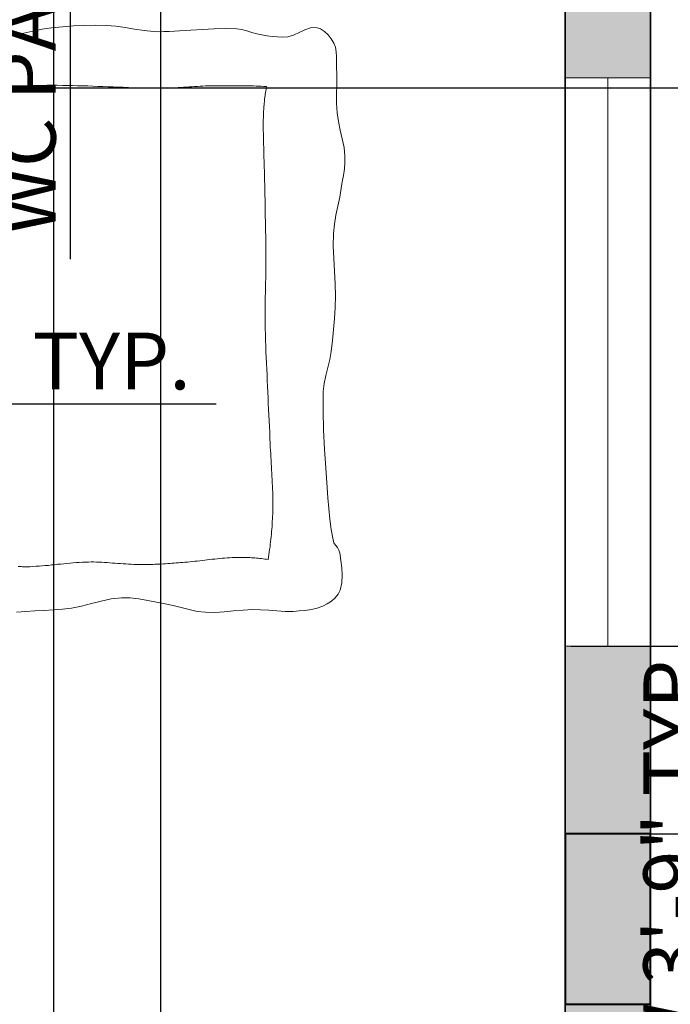
# Model space of a CAD drawing. Units: inches. Extents: x 2656 to 9931, y 1941 to 3068.
# Tile 20 of 46: x 2932 to 3000, y 2426 to 2530. Entities that reach past the tile are written whole.
import ezdxf

# ---------------------------------------------------------------- set-up
doc = ezdxf.new("R2010")
doc.units = ezdxf.units.IN
for name, color, linetype, lineweight in [('A-ANNO-DIMS', 2, 'Continuous', 18), ('A-COLS', 7, 'Continuous', 40), ('A-COLS-PATT', 146, 'Continuous', 13), ('A-FURN', 8, 'Continuous', 13), ('A-GLAZ', 4, 'Continuous', 18), ('A-WALL', 7, 'Continuous', 35), ('A-WALL-PATT', 251, 'Continuous', 13)]:
    doc.layers.add(name, color=color, linetype=linetype, lineweight=lineweight)
doc.styles.get("Standard").update_dxf_attribs({"font": 'arial.ttf'})
doc.dimstyles.new('ISO-25', dxfattribs={"dimtxt": 6, "dimasz": 2.5, "dimexe": 1.25, "dimexo": 0.625, "dimtad": 1, "dimdec": 0, "dimlunit": 3, "dimtxsty": 'Standard', "dimcen": 2.5, "dimadec": 0, "dimazin": 0, "dimtfac": 1, "dimtdec": 0, "dimtmove": 0, "dimatfit": 3, "dimfxl": 1, "dimarcsym": 0})

# ---------------------------------------------------------------- blocks, each defined once
blk = doc.blocks.new('BED-DOUBLE')
for p, q in [((54.68, 61.32), (53.7, 61.14)), ((55.65, 61.54), (54.68, 61.32)), ((56.62, 61.75), (55.65, 61.54)), ((57.61, 61.9), (56.62, 61.75)), ((58.76, 62.01), (57.61, 61.9)), ((59.92, 62.09), (58.76, 62.01)), ((61.08, 62.15), (59.92, 62.09)), ((62.25, 62.17), (61.08, 62.15)), ((63.41, 62.15), (62.25, 62.17)), ((64.4, 62.07), (63.41, 62.15)), ((65.39, 61.93), (64.4, 62.07)), ((66.38, 61.77), (65.39, 61.93)), ((67.37, 61.62), (66.38, 61.77)), ((68.37, 61.51), (67.37, 61.62)), ((68.92, 61.49), (68.37, 61.51)), ((69.47, 61.5), (68.92, 61.49)), ((70.02, 61.52), (69.47, 61.5)), ((70.57, 61.55), (70.02, 61.52)), ((71.12, 61.58), (70.57, 61.55)), ((72.32, 61.64), (71.12, 61.58)), ((73.53, 61.71), (72.32, 61.64)), ((74.74, 61.78), (73.53, 61.71)), ((75.95, 61.82), (74.74, 61.78)), ((77.16, 61.79), (75.95, 61.82)), ((77.7, 61.72), (77.16, 61.79)), ((78.23, 61.58), (77.7, 61.72)), ((78.75, 61.42), (78.23, 61.58)), ((79.28, 61.25), (78.75, 61.42)), ((83.74, 61.41), (83.15, 61.13)), ((84.33, 61.69), (83.74, 61.41)), ((84.93, 61.9), (84.33, 61.69)), ((85.54, 61.93), (84.93, 61.9)), ((86.01, 61.79), (85.54, 61.93)), ((86.43, 61.51), (86.01, 61.79)), ((86.81, 61.15), (86.43, 61.51)), ((79.82, 61.14), (79.28, 61.25)), ((80.36, 61.05), (79.82, 61.14)), ((80.9, 60.98), (80.36, 61.05)), ((81.45, 60.93), (80.9, 60.98)), ((82, 60.92), (81.45, 60.93)), ((82.54, 60.96), (82, 60.92)), ((83.15, 61.13), (82.54, 60.96)), ((87.13, 60.73), (86.81, 61.15)), ((87.4, 60.29), (87.13, 60.73)), ((87.57, 59.84), (87.4, 60.29)), ((87.66, 59.36), (87.57, 59.84)), ((87.69, 58.86), (87.66, 59.36)), ((87.69, 58.36), (87.69, 58.86)), ((87.7, 57.86), (87.69, 58.36)), ((87.72, 56.87), (87.7, 57.86)), ((87.71, 55.88), (87.72, 56.87)), ((54.6, 55.78), (54.24, 55.77)), ((54.96, 55.79), (54.6, 55.78)), ((55.33, 55.8), (54.96, 55.79)), ((55.69, 55.81), (55.33, 55.8)), ((56.05, 55.81), (55.69, 55.81)), ((56.41, 55.82), (56.05, 55.81)), ((56.77, 55.82), (56.41, 55.82)), ((57.13, 55.83), (56.77, 55.82)), ((57.49, 55.83), (57.13, 55.83)), ((57.85, 55.83), (57.49, 55.83)), ((58.21, 55.83), (57.85, 55.83)), ((58.75, 55.82), (58.21, 55.83)), ((59.28, 55.81), (58.75, 55.82)), ((59.82, 55.8), (59.28, 55.81)), ((60.36, 55.79), (59.82, 55.8)), ((60.89, 55.77), (60.36, 55.79)), ((61.43, 55.76), (60.89, 55.77)), ((61.96, 55.74), (61.43, 55.76)), ((62.5, 55.72), (61.96, 55.74)), ((63.04, 55.7), (62.5, 55.72)), ((63.57, 55.68), (63.04, 55.7)), ((64.11, 55.66), (63.57, 55.68)), ((64.65, 55.64), (64.11, 55.66)), ((65.18, 55.62), (64.65, 55.64)), ((65.72, 55.6), (65.18, 55.62)), ((66.25, 55.58), (65.72, 55.6)), ((66.79, 55.57), (66.25, 55.58)), ((67.33, 55.56), (66.79, 55.57)), ((67.86, 55.55), (67.33, 55.56)), ((68.4, 55.54), (67.86, 55.55)), ((68.94, 55.54), (68.4, 55.54)), ((69.23, 55.54), (68.94, 55.54)), ((69.52, 55.54), (69.23, 55.54)), ((69.81, 55.55), (69.52, 55.54)), ((70.1, 55.56), (69.81, 55.55)), ((70.39, 55.57), (70.1, 55.56)), ((70.68, 55.58), (70.39, 55.57)), ((70.97, 55.6), (70.68, 55.58)), ((71.26, 55.61), (70.97, 55.6)), ((71.55, 55.63), (71.26, 55.61)), ((71.84, 55.65), (71.55, 55.63)), ((72.13, 55.66), (71.84, 55.65)), ((72.42, 55.68), (72.13, 55.66)), ((72.71, 55.7), (72.42, 55.68)), ((73, 55.72), (72.71, 55.7)), ((73.29, 55.73), (73, 55.72)), ((73.58, 55.75), (73.29, 55.73)), ((73.87, 55.76), (73.58, 55.75)), ((74.16, 55.77), (73.87, 55.76)), ((74.45, 55.78), (74.16, 55.77)), ((74.74, 55.78), (74.45, 55.78)), ((75.01, 55.79), (74.74, 55.78)), ((75.29, 55.79), (75.01, 55.79)), ((75.57, 55.79), (75.29, 55.79)), ((75.85, 55.79), (75.57, 55.79)), ((76.13, 55.79), (75.85, 55.79)), ((76.41, 55.79), (76.13, 55.79)), ((76.68, 55.79), (76.41, 55.79)), ((76.96, 55.79), (76.68, 55.79)), ((77.24, 55.79), (76.96, 55.79)), ((77.52, 55.79), (77.24, 55.79)), ((77.8, 55.78), (77.52, 55.79)), ((78.08, 55.78), (77.8, 55.78)), ((78.36, 55.77), (78.08, 55.78)), ((78.63, 55.77), (78.36, 55.77)), ((78.91, 55.76), (78.63, 55.77)), ((79.19, 55.75), (78.91, 55.76)), ((79.47, 55.74), (79.19, 55.75)), ((79.75, 55.73), (79.47, 55.74)), ((80.03, 55.72), (79.75, 55.73)), ((80.3, 55.71), (80.03, 55.72)), ((80.17, 54.91), (80.19, 55.07)), ((80.19, 55.07), (80.22, 55.23)), ((80.22, 55.23), (80.25, 55.39)), ((80.25, 55.39), (80.27, 55.55)), ((80.27, 55.55), (80.3, 55.71)), ((87.69, 54.89), (87.71, 55.88)), ((80.05, 53.94), (80.07, 54.1)), ((80.07, 54.1), (80.09, 54.26)), ((80.09, 54.26), (80.1, 54.42)), ((80.1, 54.42), (80.13, 54.59)), ((80.13, 54.59), (80.15, 54.75)), ((80.15, 54.75), (80.17, 54.91)), ((87.69, 53.9), (87.69, 54.89)), ((79.99, 53.13), (80, 53.29)), ((79.99, 52.96), (79.99, 53.13)), ((80, 53.29), (80.01, 53.45)), ((80.01, 53.45), (80.02, 53.61)), ((80.02, 53.61), (80.04, 53.78)), ((80.04, 53.78), (80.05, 53.94)), ((87.75, 52.91), (87.69, 53.9)), ((79.96, 52.12), (79.97, 52.47)), ((79.96, 51.76), (79.96, 52.12)), ((79.97, 52.64), (79.98, 52.8)), ((79.97, 52.47), (79.97, 52.64)), ((79.98, 52.8), (79.99, 52.96)), ((87.88, 52), (87.75, 52.91)), ((88.08, 51.09), (87.88, 52)), ((79.96, 51.41), (79.96, 51.76)), ((79.96, 51.05), (79.96, 51.41)), ((79.97, 50.7), (79.96, 51.05)), ((88.29, 50.19), (88.08, 51.09)), ((79.97, 50.34), (79.97, 50.7)), ((79.98, 49.99), (79.97, 50.34)), ((79.99, 49.63), (79.98, 49.99)), ((88.48, 49.28), (88.29, 50.19)), ((80, 49.28), (79.99, 49.63)), ((80.01, 48.92), (80, 49.28)), ((80.02, 48.57), (80.01, 48.92)), ((88.58, 48.36), (88.48, 49.28)), ((80.03, 48.21), (80.02, 48.57)), ((80.04, 47.85), (80.03, 48.21)), ((80.05, 47.5), (80.04, 47.85)), ((88.58, 47.69), (88.58, 48.36)), ((80.06, 47.14), (80.05, 47.5)), ((80.07, 46.79), (80.06, 47.14)), ((80.08, 46.43), (80.07, 46.79)), ((88.41, 46.33), (88.52, 47.01)), ((88.52, 47.01), (88.58, 47.69)), ((80.09, 46.08), (80.08, 46.43)), ((80.1, 45.72), (80.09, 46.08)), ((80.11, 45.37), (80.1, 45.72)), ((88.29, 45.66), (88.41, 46.33)), ((80.12, 44.98), (80.11, 45.37)), ((80.12, 44.6), (80.12, 44.98)), ((88.02, 44.03), (88.18, 44.99)), ((88.18, 44.99), (88.29, 45.66)), ((80.13, 44.21), (80.12, 44.6)), ((80.14, 43.83), (80.13, 44.21)), ((80.14, 43.44), (80.14, 43.83)), ((87.82, 43.07), (88.02, 44.03)), ((80.15, 43.06), (80.14, 43.44)), ((80.16, 42.67), (80.15, 43.06)), ((80.17, 42.29), (80.16, 42.67)), ((87.63, 42.12), (87.82, 43.07)), ((80.17, 41.9), (80.17, 42.29)), ((80.18, 41.52), (80.17, 41.9)), ((87.47, 41.16), (87.63, 42.12)), ((80.19, 41.14), (80.18, 41.52)), ((80.19, 40.75), (80.19, 41.14)), ((80.2, 40.37), (80.19, 40.75)), ((87.37, 40.19), (87.47, 41.16)), ((80.21, 39.98), (80.2, 40.37)), ((80.21, 39.6), (80.21, 39.98)), ((80.22, 39.21), (80.21, 39.6)), ((87.35, 38.87), (87.37, 40.19)), ((80.22, 38.83), (80.22, 39.21)), ((80.22, 38.44), (80.22, 38.83)), ((87.4, 37.54), (87.35, 38.87)), ((80.23, 38.06), (80.22, 38.44)), ((80.23, 37.67), (80.23, 38.06)), ((80.23, 37.3), (80.23, 37.67)), ((87.48, 36.22), (87.4, 37.54)), ((80.22, 36.54), (80.23, 36.92)), ((80.22, 36.17), (80.22, 36.54)), ((80.23, 36.92), (80.23, 37.3)), ((80.2, 35.04), (80.21, 35.42)), ((80.21, 35.79), (80.22, 36.17)), ((80.21, 35.42), (80.21, 35.79)), ((87.55, 34.89), (87.48, 36.22)), ((80.19, 34.66), (80.2, 35.04)), ((80.19, 34.29), (80.19, 34.66)), ((87.57, 33.57), (87.55, 34.89)), ((80.17, 33.53), (80.18, 33.91)), ((80.17, 33.16), (80.17, 33.53)), ((80.18, 33.91), (80.19, 34.29)), ((87.53, 32.4), (87.57, 33.57)), ((80.16, 32.78), (80.17, 33.16)), ((80.16, 32.41), (80.16, 32.78)), ((80.16, 32.03), (80.16, 32.41)), ((87.47, 31.23), (87.53, 32.4)), ((80.15, 31.65), (80.16, 32.03)), ((80.15, 31.28), (80.15, 31.65)), ((80.16, 30.9), (80.15, 31.28)), ((87.38, 30.07), (87.47, 31.23)), ((80.16, 30.52), (80.16, 30.9)), ((80.17, 30.15), (80.16, 30.52)), ((80.19, 29.54), (80.17, 30.15)), ((80.2, 28.93), (80.19, 29.54)), ((87.26, 28.91), (87.38, 30.07)), ((80.22, 28.32), (80.2, 28.93)), ((80.24, 27.71), (80.22, 28.32)), ((87.13, 27.75), (87.26, 28.91)), ((80.27, 27.11), (80.24, 27.71)), ((80.29, 26.5), (80.27, 27.11)), ((86.97, 26.9), (87.13, 27.75)), ((80.32, 25.89), (80.29, 26.5)), ((86.55, 25.22), (86.76, 26.06)), ((86.76, 26.06), (86.97, 26.9)), ((80.35, 25.28), (80.32, 25.89)), ((80.37, 24.67), (80.35, 25.28)), ((86.37, 24.38), (86.55, 25.22)), ((80.4, 24.06), (80.37, 24.67)), ((80.43, 23.46), (80.4, 24.06)), ((86.28, 23.52), (86.37, 24.38)), ((80.46, 22.85), (80.43, 23.46)), ((86.27, 21.49), (86.28, 23.52)), ((80.49, 22.24), (80.46, 22.85)), ((80.52, 21.63), (80.49, 22.24)), ((80.55, 21.02), (80.52, 21.63)), ((80.58, 20.41), (80.55, 21.02)), ((86.32, 19.47), (86.27, 21.49)), ((80.61, 19.81), (80.58, 20.41)), ((80.64, 19.2), (80.61, 19.81)), ((80.66, 18.59), (80.64, 19.2)), ((86.43, 17.44), (86.32, 19.47)), ((80.69, 17.98), (80.66, 18.59)), ((80.7, 17.64), (80.69, 17.98)), ((80.72, 17.3), (80.7, 17.64)), ((80.74, 16.96), (80.72, 17.3)), ((80.76, 16.62), (80.74, 16.96)), ((86.56, 15.42), (86.43, 17.44)), ((80.78, 16.27), (80.76, 16.62)), ((80.8, 15.93), (80.78, 16.27)), ((80.82, 15.59), (80.8, 15.93)), ((80.84, 15.25), (80.82, 15.59)), ((80.86, 14.91), (80.84, 15.25)), ((80.87, 14.57), (80.86, 14.91)), ((80.89, 14.23), (80.87, 14.57)), ((86.7, 13.4), (86.56, 15.42)), ((80.91, 13.88), (80.89, 14.23)), ((80.92, 13.54), (80.91, 13.88)), ((80.94, 13.2), (80.92, 13.54)), ((80.95, 12.86), (80.94, 13.2)), ((80.96, 12.52), (80.95, 12.86)), ((80.96, 12.18), (80.96, 12.52)), ((86.78, 12.28), (86.7, 13.4)), ((80.96, 11.84), (80.96, 12.18)), ((80.96, 11.49), (80.96, 11.84)), ((80.96, 11.15), (80.96, 11.49)), ((86.87, 11.17), (86.78, 12.28)), ((80.94, 10.34), (80.95, 10.61)), ((80.95, 10.88), (80.96, 11.15)), ((80.95, 10.61), (80.95, 10.88)), ((86.98, 10.05), (86.87, 11.17)), ((80.88, 9.26), (80.89, 9.53)), ((80.89, 9.53), (80.91, 9.8)), ((80.91, 9.8), (80.92, 10.07)), ((80.92, 10.07), (80.94, 10.34)), ((87.13, 8.95), (86.98, 10.05)), ((80.79, 8.19), (80.81, 8.46)), ((80.81, 8.46), (80.84, 8.73)), ((80.84, 8.73), (80.86, 9)), ((80.86, 9), (80.88, 9.26)), ((87.32, 7.85), (87.13, 8.95)), ((80.67, 7.12), (80.7, 7.38)), ((80.7, 7.38), (80.73, 7.65)), ((80.73, 7.65), (80.76, 7.92)), ((80.76, 7.92), (80.79, 8.19)), ((87.42, 7.56), (87.32, 7.85)), ((87.59, 7.3), (87.42, 7.56)), ((87.78, 7.04), (87.59, 7.3)), ((80.51, 6.05), (80.56, 6.31)), ((80.56, 6.31), (80.59, 6.58)), ((80.59, 6.58), (80.63, 6.85)), ((80.63, 6.85), (80.67, 7.12)), ((87.94, 6.78), (87.78, 7.04)), ((88.04, 6.49), (87.94, 6.78)), ((88.15, 5.7), (88.04, 6.49)), ((57.28, 5.17), (57.6, 5.21)), ((57.6, 5.21), (57.93, 5.24)), ((57.93, 5.24), (58.26, 5.28)), ((58.26, 5.28), (58.58, 5.31)), ((58.58, 5.31), (58.91, 5.34)), ((58.91, 5.34), (59.23, 5.38)), ((59.23, 5.38), (59.56, 5.41)), ((59.56, 5.41), (59.88, 5.44)), ((59.88, 5.44), (60.21, 5.46)), ((60.21, 5.46), (60.53, 5.48)), ((60.53, 5.48), (60.86, 5.5)), ((60.86, 5.5), (61.19, 5.52)), ((61.19, 5.52), (61.51, 5.52)), ((61.51, 5.52), (61.8, 5.53)), ((61.8, 5.53), (62.08, 5.53)), ((62.08, 5.53), (62.36, 5.52)), ((62.36, 5.52), (62.64, 5.51)), ((62.64, 5.51), (62.92, 5.5)), ((62.92, 5.5), (63.21, 5.48)), ((63.21, 5.48), (63.49, 5.46)), ((63.49, 5.46), (63.77, 5.44)), ((63.77, 5.44), (64.05, 5.42)), ((64.05, 5.42), (64.33, 5.4)), ((64.33, 5.4), (64.62, 5.38)), ((64.62, 5.38), (64.9, 5.36)), ((64.9, 5.36), (65.18, 5.34)), ((65.18, 5.34), (65.46, 5.32)), ((65.46, 5.32), (65.74, 5.3)), ((65.74, 5.3), (66.03, 5.28)), ((66.03, 5.28), (66.31, 5.27)), ((66.31, 5.27), (66.59, 5.26)), ((66.59, 5.26), (66.87, 5.25)), ((66.87, 5.25), (67.15, 5.25)), ((67.15, 5.25), (67.38, 5.25)), ((67.38, 5.25), (67.61, 5.25)), ((67.61, 5.25), (67.83, 5.26)), ((67.83, 5.26), (68.06, 5.26)), ((68.06, 5.26), (68.29, 5.27)), ((68.29, 5.27), (68.51, 5.28)), ((68.51, 5.28), (68.74, 5.29)), ((68.74, 5.29), (68.97, 5.3)), ((68.97, 5.3), (69.19, 5.31)), ((69.19, 5.31), (69.42, 5.33)), ((69.42, 5.33), (69.65, 5.34)), ((69.65, 5.34), (69.87, 5.36)), ((69.87, 5.36), (70.1, 5.38)), ((70.1, 5.38), (70.33, 5.39)), ((70.33, 5.39), (70.55, 5.41)), ((70.55, 5.41), (70.78, 5.43)), ((70.78, 5.43), (71, 5.44)), ((71, 5.44), (71.23, 5.46)), ((71.23, 5.46), (71.46, 5.48)), ((71.46, 5.48), (71.68, 5.5)), ((71.68, 5.5), (71.95, 5.52)), ((71.95, 5.52), (72.21, 5.54)), ((72.21, 5.54), (72.47, 5.57)), ((72.47, 5.57), (72.73, 5.6)), ((72.73, 5.6), (72.99, 5.63)), ((72.99, 5.63), (73.26, 5.66)), ((73.26, 5.66), (73.52, 5.69)), ((73.52, 5.69), (73.78, 5.72)), ((73.78, 5.72), (74.04, 5.75)), ((74.04, 5.75), (74.3, 5.78)), ((74.3, 5.78), (74.57, 5.81)), ((74.57, 5.81), (74.83, 5.84)), ((74.83, 5.84), (75.09, 5.87)), ((75.09, 5.87), (75.35, 5.89)), ((75.35, 5.89), (75.61, 5.92)), ((75.61, 5.92), (75.88, 5.94)), ((75.88, 5.94), (76.14, 5.96)), ((76.14, 5.96), (76.4, 5.98)), ((76.4, 5.98), (76.66, 5.99)), ((76.66, 5.99), (76.93, 6)), ((76.93, 6), (77.1, 6.01)), ((77.1, 6.01), (77.28, 6.01)), ((77.28, 6.01), (77.46, 6.01)), ((77.46, 6.01), (77.64, 6.01)), ((77.64, 6.01), (77.82, 6.01)), ((77.82, 6.01), (77.99, 6.01)), ((77.99, 6.01), (78.17, 6)), ((78.17, 6), (78.35, 5.99)), ((78.35, 5.99), (78.53, 5.99)), ((78.53, 5.99), (78.7, 5.98)), ((78.7, 5.98), (78.88, 5.96)), ((78.88, 5.96), (79.06, 5.95)), ((79.06, 5.95), (79.24, 5.93)), ((79.24, 5.93), (79.41, 5.92)), ((79.41, 5.92), (79.59, 5.9)), ((79.59, 5.9), (79.77, 5.88)), ((79.77, 5.88), (79.94, 5.86)), ((79.94, 5.86), (80.12, 5.83)), ((80.12, 5.83), (80.3, 5.81)), ((80.3, 5.81), (80.47, 5.78)), ((80.47, 5.78), (80.51, 6.05)), ((88.24, 4.91), (88.15, 5.7)), ((54.1, 5.06), (54.25, 5.05)), ((54.25, 5.05), (54.4, 5.04)), ((54.4, 5.04), (54.55, 5.03)), ((54.55, 5.03), (54.7, 5.02)), ((54.7, 5.02), (54.85, 5.02)), ((54.85, 5.02), (55, 5.02)), ((55, 5.02), (55.32, 5.03)), ((55.32, 5.03), (55.65, 5.05)), ((55.65, 5.05), (55.98, 5.07)), ((55.98, 5.07), (56.3, 5.09)), ((56.3, 5.09), (56.63, 5.11)), ((56.63, 5.11), (56.95, 5.14)), ((56.95, 5.14), (57.28, 5.17)), ((88.28, 4.12), (88.24, 4.91)), ((88.06, 2.57), (88.23, 3.33)), ((88.23, 3.33), (88.28, 4.12)), ((87.53, 1.73), (87.85, 2.13)), ((87.85, 2.13), (88.06, 2.57)), ((60.77, 0.87), (61.82, 1.13)), ((61.82, 1.13), (62.86, 1.41)), ((62.86, 1.41), (63.92, 1.63)), ((63.92, 1.63), (64.98, 1.75)), ((64.98, 1.75), (65.91, 1.74)), ((65.91, 1.74), (66.84, 1.63)), ((66.84, 1.63), (67.76, 1.47)), ((67.76, 1.47), (68.68, 1.29)), ((68.68, 1.29), (69.6, 1.11)), ((69.6, 1.11), (70.45, 0.93)), ((86.25, 0.88), (86.7, 1.11)), ((86.7, 1.11), (87.14, 1.4)), ((87.14, 1.4), (87.53, 1.73)), ((53.91, 0.24), (54.88, 0.3)), ((54.88, 0.3), (55.85, 0.36)), ((55.85, 0.36), (56.82, 0.41)), ((56.82, 0.41), (57.79, 0.47)), ((57.79, 0.47), (58.75, 0.55)), ((58.75, 0.55), (59.72, 0.66)), ((59.72, 0.66), (60.77, 0.87)), ((70.45, 0.93), (71.29, 0.72)), ((71.29, 0.72), (72.14, 0.5)), ((72.14, 0.5), (72.99, 0.32)), ((72.99, 0.32), (73.85, 0.22)), ((73.85, 0.22), (74.84, 0.2)), ((74.84, 0.2), (75.84, 0.27)), ((75.84, 0.27), (76.83, 0.37)), ((76.83, 0.37), (77.83, 0.46)), ((77.83, 0.46), (78.82, 0.51)), ((78.82, 0.51), (79.68, 0.49)), ((79.68, 0.49), (80.54, 0.43)), ((80.54, 0.43), (81.39, 0.36)), ((81.39, 0.36), (82.25, 0.32)), ((82.25, 0.32), (83.1, 0.32)), ((83.1, 0.32), (83.75, 0.36)), ((83.75, 0.36), (84.39, 0.41)), ((84.39, 0.41), (85.03, 0.51)), ((85.03, 0.51), (85.65, 0.66)), ((85.65, 0.66), (86.25, 0.88))]:
    blk.add_line(p, q)
blk = doc.blocks.new('WIN-60IN-SASH')
for p, q in [((4.46, 60.03), (-0.04, 60.03)), ((4.46, 0.03), (4.46, 60.03))]:
    blk.add_line(p, q)
blk = doc.blocks.new('*D29')
at = {"layer": 'A-ANNO-DIMS', "color": 0, "lineweight": -2, "transparency": 16777216}
for p, q in [((2939.24, 2614.86), (2935.66, 2614.86)), ((2936.91, 2612.36), (2936.91, 2597.65)), ((2939.24, 2595.15), (2935.66, 2595.15)), ((2936.91, 2595.15), (2936.91, 2504.75))]:
    blk.add_line(p, q, dxfattribs=at)
at = {"layer": 'A-ANNO-DIMS', "color": 0, "transparency": 16777216}
for points in [[(2936.49, 2612.36), (2937.33, 2612.36), (2936.91, 2614.86)], [(2936.49, 2597.65), (2937.33, 2597.65), (2936.91, 2595.15)]]:
    blk.add_solid(points, dxfattribs=at)
at = {"layer": 'Defpoints', "color": 0, "transparency": 16777216}
for p in [(2939.87, 2614.86), (2936.91, 2595.15), (2939.87, 2595.15)]:
    blk.add_point(p, dxfattribs=at)
at = {"layer": 'A-ANNO-DIMS', "color": 0, "transparency": 16777216, "insert": (2933.18, 2548.7), "char_height": 6, "attachment_point": 5, "rotation": 90}
blk.add_mtext('WC PAN 1\'-7 1/2" TYP.', dxfattribs=at)
blk = doc.blocks.new('*D31')
at = {"layer": 'A-ANNO-DIMS', "color": 0, "lineweight": -2, "transparency": 16777216}
for p, q in [((2753.36, 2502.15), (2753.36, 2488.23)), ((2841.98, 2502.15), (2841.98, 2488.23)), ((2755.86, 2489.48), (2839.48, 2489.48)), ((2841.98, 2489.48), (2952.35, 2489.48))]:
    blk.add_line(p, q, dxfattribs=at)
at = {"layer": 'A-ANNO-DIMS', "color": 0, "transparency": 16777216}
for points in [[(2755.86, 2489.89), (2755.86, 2489.06), (2753.36, 2489.48)], [(2839.48, 2489.89), (2839.48, 2489.06), (2841.98, 2489.48)]]:
    blk.add_solid(points, dxfattribs=at)
at = {"layer": 'Defpoints', "color": 0, "transparency": 16777216}
for p in [(2753.36, 2502.77), (2841.98, 2502.77), (2841.98, 2489.48)]:
    blk.add_point(p, dxfattribs=at)
at = {"layer": 'A-ANNO-DIMS', "color": 0, "transparency": 16777216, "insert": (2898.41, 2493.21), "char_height": 6, "attachment_point": 5}
blk.add_mtext('DOUBLE BED 7\'-4 1/2" TYP.', dxfattribs=at)
blk = doc.blocks.new('*D47')
at = {"layer": 'A-ANNO-DIMS', "color": 0, "lineweight": -2, "transparency": 16777216}
for p, q in [((3004.93, 2365.04), (3004.93, 2467.44)), ((2998.78, 2365.04), (3006.18, 2365.04)), ((3004.93, 2322.38), (3004.93, 2362.54)), ((2998.78, 2319.88), (3006.18, 2319.88))]:
    blk.add_line(p, q, dxfattribs=at)
at = {"layer": 'A-ANNO-DIMS', "color": 0, "transparency": 16777216}
for points in [[(3004.51, 2362.54), (3005.35, 2362.54), (3004.93, 2365.04)], [(3004.51, 2322.38), (3005.35, 2322.38), (3004.93, 2319.88)]]:
    blk.add_solid(points, dxfattribs=at)
at = {"layer": 'Defpoints', "color": 0, "transparency": 16777216}
for p in [(2998.16, 2365.04), (3004.93, 2365.04), (2998.16, 2319.88)]:
    blk.add_point(p, dxfattribs=at)
at = {"layer": 'A-ANNO-DIMS', "color": 0, "transparency": 16777216, "insert": (3001.2, 2417.49), "char_height": 6, "attachment_point": 5, "rotation": 90}
blk.add_mtext('HALL WINDOW 3\'-9" TYP.', dxfattribs=at)
blk = doc.blocks.new('*D75')
at = {"layer": 'A-ANNO-DIMS', "color": 0, "lineweight": -2, "transparency": 16777216}
for p, q in [((2989.78, 2463.88), (3061.01, 2463.88)), ((3059.76, 2446.6), (3059.76, 2461.38)), ((2989.78, 2444.1), (3061.01, 2444.1))]:
    blk.add_line(p, q, dxfattribs=at)
at = {"layer": 'A-ANNO-DIMS', "color": 0, "transparency": 16777216}
for points in [[(3059.34, 2461.38), (3060.17, 2461.38), (3059.76, 2463.88)], [(3059.34, 2446.6), (3060.17, 2446.6), (3059.76, 2444.1)]]:
    blk.add_solid(points, dxfattribs=at)
at = {"layer": 'Defpoints', "color": 0, "transparency": 16777216}
for p in [(2989.16, 2463.88), (3059.76, 2463.88), (2989.16, 2444.1)]:
    blk.add_point(p, dxfattribs=at)
at = {"layer": 'A-ANNO-DIMS', "color": 0, "transparency": 16777216, "insert": (3056.07, 2453.99), "char_height": 6, "attachment_point": 5, "rotation": 90}
blk.add_mtext('1\'-8"', dxfattribs=at)
blk = doc.blocks.new('*D101')
at = {"layer": 'A-ANNO-DIMS', "color": 0, "lineweight": -2, "transparency": 16777216}
for p, q in [((2935.16, 2553.98), (2935.16, 2009.27)), ((2946.47, 2553.98), (2946.47, 2009.27)), ((2937.66, 2010.52), (2943.97, 2010.52)), ((2946.47, 2010.52), (2984.81, 2010.52))]:
    blk.add_line(p, q, dxfattribs=at)
at = {"layer": 'A-ANNO-DIMS', "color": 0, "transparency": 16777216}
for points in [[(2937.66, 2010.94), (2937.66, 2010.11), (2935.16, 2010.52)], [(2943.97, 2010.94), (2943.97, 2010.11), (2946.47, 2010.52)]]:
    blk.add_solid(points, dxfattribs=at)
at = {"layer": 'Defpoints', "color": 0, "transparency": 16777216}
for p in [(2935.16, 2554.6), (2946.47, 2554.6), (2946.47, 2010.52)]:
    blk.add_point(p, dxfattribs=at)
at = {"layer": 'A-ANNO-DIMS', "color": 0, "transparency": 16777216, "insert": (2966.89, 2014.25), "char_height": 6, "attachment_point": 5}
blk.add_mtext('0\'-11 1/2"', dxfattribs=at)
blk = doc.blocks.new('*D102')
at = {"layer": 'A-ANNO-DIMS', "color": 0, "lineweight": -2, "transparency": 16777216}
for p, q in [((2998.16, 2604.98), (2998.16, 2009.27)), ((2872.16, 2564.71), (2872.16, 2009.27)), ((2874.66, 2010.52), (2995.66, 2010.52))]:
    blk.add_line(p, q, dxfattribs=at)
at = {"layer": 'A-ANNO-DIMS', "color": 0, "transparency": 16777216}
for points in [[(2874.66, 2010.94), (2874.66, 2010.11), (2872.16, 2010.52)], [(2995.66, 2010.94), (2995.66, 2010.11), (2998.16, 2010.52)]]:
    blk.add_solid(points, dxfattribs=at)
at = {"layer": 'Defpoints', "color": 0, "transparency": 16777216}
for p in [(2998.16, 2605.6), (2872.16, 2565.34), (2998.16, 2010.52)]:
    blk.add_point(p, dxfattribs=at)
at = {"layer": 'A-ANNO-DIMS', "color": 0, "transparency": 16777216, "insert": (2935.16, 2014.21), "char_height": 6, "attachment_point": 5}
blk.add_mtext('10\'-6"', dxfattribs=at)
blk = doc.blocks.new('*D130')
at = {"layer": 'A-ANNO-DIMS', "color": 0, "lineweight": -2, "transparency": 16777216}
for p, q in [((2877.28, 2538.52), (3061.01, 2538.52)), ((3059.76, 2536.02), (3059.76, 2525.32)), ((2902.17, 2522.82), (3061.01, 2522.82)), ((3059.76, 2522.82), (3059.76, 2489.7))]:
    blk.add_line(p, q, dxfattribs=at)
at = {"layer": 'A-ANNO-DIMS', "color": 0, "transparency": 16777216}
for points in [[(3059.34, 2536.02), (3060.17, 2536.02), (3059.76, 2538.52)], [(3059.34, 2525.32), (3060.17, 2525.32), (3059.76, 2522.82)]]:
    blk.add_solid(points, dxfattribs=at)
at = {"layer": 'Defpoints', "color": 0, "transparency": 16777216}
for p in [(2876.66, 2538.52), (2901.54, 2522.82), (3059.76, 2522.82)]:
    blk.add_point(p, dxfattribs=at)
at = {"layer": 'A-ANNO-DIMS', "color": 0, "transparency": 16777216, "insert": (3056.03, 2505.01), "char_height": 6, "attachment_point": 5, "rotation": 90}
blk.add_mtext('1\'-3 1/2"', dxfattribs=at)

msp = doc.modelspace()

# ---------------------------------------------------------------- hatches: boundary and pattern name
at = {"layer": 'A-COLS-PATT'}
h = msp.add_hatch(color=256, dxfattribs=at)
h.dxf.hatch_style = 1
h.paths.add_polyline_path([(2752.16, 2623.6), (2743.16, 2623.6), (2743.16, 2605.6), (2752.16, 2605.6)])
h.paths.add_polyline_path([(2876.66, 2623.6), (2858.66, 2623.6), (2858.66, 2614.6), (2876.66, 2614.6)])
h.paths.add_polyline_path([(2998.16, 2623.6), (2989.16, 2623.6), (2989.16, 2614.6), (2989.16, 2605.6), (2998.16, 2605.6)])
h.paths.add_polyline_path([(2998.16, 2444.1), (2989.16, 2444.1), (2989.16, 2426.1), (2998.16, 2426.1)])
h.paths.add_polyline_path([(2876.66, 2444.1), (2867.66, 2444.1), (2867.66, 2426.1), (2876.66, 2426.1)])
h.paths.add_polyline_path([(2752.16, 2444.1), (2743.16, 2444.1), (2743.16, 2426.1), (2752.16, 2426.1)])
h.paths.add_polyline_path([(2752.16, 2300.1), (2743.16, 2300.1), (2743.16, 2282.1), (2752.16, 2282.1)])
h.paths.add_polyline_path([(2876.66, 2300.1), (2867.66, 2300.1), (2867.66, 2282.1), (2876.66, 2282.1)])
h.paths.add_polyline_path([(2998.16, 2300.1), (2989.16, 2300.1), (2989.16, 2282.1), (2998.16, 2282.1)])
h.paths.add_polyline_path([(2998.16, 2184.6), (2989.16, 2184.6), (2989.16, 2166.6), (2998.16, 2166.6)])
h.paths.add_polyline_path([(2876.66, 2175.6), (2858.66, 2175.6), (2858.66, 2166.6), (2876.66, 2166.6)])
h.paths.add_polyline_path([(2752.16, 2184.6), (2743.16, 2184.6), (2743.16, 2166.6), (2752.16, 2166.6)])
at = {"layer": 'A-WALL-PATT'}
h = msp.add_hatch(color=256, dxfattribs=at)
h.dxf.hatch_style = 1
h.paths.add_polyline_path([(2858.66, 2623.6), (2752.16, 2623.6), (2752.16, 2614.6), (2858.66, 2614.6)])
h.paths.add_polyline_path([(2893.09, 2623.6), (2876.66, 2623.6), (2876.66, 2614.6), (2893.09, 2614.6), (2893.09, 2619.1)])
h.paths.add_polyline_path([(2946.51, 2623.6), (2917.09, 2623.6), (2917.09, 2614.6), (2946.51, 2614.6), (2946.51, 2619.1)])
h.paths.add_polyline_path([(2989.16, 2623.6), (2970.51, 2623.6), (2970.51, 2614.6), (2989.16, 2614.6)])
h.paths.add_polyline_path([(2998.16, 2605.6), (2989.16, 2605.6), (2989.16, 2523.88), (2998.16, 2523.88)])
h.paths.add_polyline_path([(2935.16, 2614.6), (2930.66, 2614.6), (2930.66, 2554.6), (2876.66, 2554.6), (2876.66, 2565.34), (2872.16, 2565.34), (2872.16, 2444.1), (2876.66, 2444.1), (2876.66, 2550.1), (2946.47, 2550.1), (2946.47, 2554.6), (2935.16, 2554.6)])
h.paths.add_polyline_path([(2989.16, 2554.6), (2982.11, 2554.6), (2976.57, 2554.6), (2976.57, 2550.1), (2982.11, 2550.1), (2989.16, 2550.1)])
h.paths.add_polyline_path([(2876.66, 2614.6), (2872.16, 2614.6), (2872.16, 2595), (2876.66, 2595)], flags=0)
h.paths.add_polyline_path([(2752.16, 2605.6), (2743.16, 2605.6), (2743.16, 2544.03), (2752.16, 2544.03)])
h.paths.add_polyline_path([(2752.16, 2426.1), (2743.16, 2426.1), (2743.16, 2300.1), (2752.16, 2300.1)])
h.paths.add_polyline_path([(2821.13, 2430.6), (2752.16, 2430.6), (2752.16, 2426.1), (2821.13, 2426.1)])
h.paths.add_polyline_path([(2867.66, 2430.6), (2862.88, 2430.6), (2862.88, 2426.1), (2867.66, 2426.1)])
h.paths.add_polyline_path([(2752.16, 2484.03), (2747.66, 2484.03), (2743.16, 2484.03), (2743.16, 2444.1), (2752.16, 2444.1)])
h.paths.add_polyline_path([(2998.16, 2426.1), (2989.16, 2426.1), (2989.16, 2390.1), (2872.16, 2390.1), (2872.16, 2385.6), (2876.66, 2385.6), (2989.16, 2385.6), (2989.16, 2365.04), (2998.16, 2365.04)])
h.paths.add_polyline_path([(2998.16, 2463.88), (2993.66, 2463.88), (2989.16, 2463.88), (2989.16, 2444.1), (2998.16, 2444.1)])
h.paths.add_polyline_path([(2998.16, 2319.88), (2989.16, 2319.88), (2989.16, 2300.1), (2998.16, 2300.1)])
h.paths.add_polyline_path([(2998.16, 2282.1), (2989.16, 2282.1), (2989.16, 2253.6), (2982.06, 2253.6), (2982.06, 2249.1), (2989.16, 2249.1), (2998.16, 2249.1)])
h.paths.add_polyline_path([(2931.54, 2253.6), (2923.8, 2253.6), (2923.8, 2249.1), (2931.54, 2249.1)])
h.paths.add_polyline_path([(2876.66, 2282.1), (2872.16, 2282.1), (2872.16, 2184.6), (2872.16, 2175.6), (2876.66, 2175.6), (2876.66, 2249.1), (2888.32, 2249.1), (2888.32, 2251.35), (2888.32, 2253.6), (2876.66, 2253.6)])
h.paths.add_polyline_path([(2858.66, 2175.6), (2841.42, 2175.6), (2841.42, 2166.6), (2858.66, 2166.6)])
h.paths.add_polyline_path([(2785.06, 2171.1), (2785.06, 2175.6), (2752.16, 2175.6), (2752.16, 2166.6), (2785.06, 2166.6)])
h.paths.add_polyline_path([(2752.16, 2282.1), (2743.16, 2282.1), (2743.16, 2184.6), (2752.16, 2184.6)])
h.paths.add_polyline_path([(2809.77, 2300.1), (2752.16, 2300.1), (2752.16, 2295.6), (2809.77, 2295.6)])
h.paths.add_polyline_path([(2867.66, 2300.1), (2851.88, 2300.1), (2851.88, 2295.6), (2867.66, 2295.6)])

# ---------------------------------------------------------------- linework, layer by layer
at = {"layer": 'A-COLS'}
for p, q in [((2998.16, 2444.1), (2989.16, 2444.1)), ((2989.16, 2444.1), (2989.16, 2444.1)), ((2989.16, 2444.1), (2989.16, 2426.1)), ((2998.16, 2426.1), (2998.16, 2444.1)), ((2989.16, 2426.1), (2998.16, 2426.1))]:
    msp.add_line(p, q, dxfattribs=at)
at = {"layer": 'A-GLAZ'}
for p, q in [((2989.16, 2523.88), (2998.16, 2523.88)), ((2989.16, 2463.88), (2998.16, 2463.88)), ((2998.16, 2463.88), (2993.66, 2463.88))]:
    msp.add_line(p, q, dxfattribs=at)
at = {"layer": 'A-WALL'}
for p, q in [((2998.16, 2623.6), (2998.16, 2249.1)), ((2989.16, 2614.6), (2989.16, 2390.1))]:
    msp.add_line(p, q, dxfattribs=at)

# ---------------------------------------------------------------- block references
at = {"layer": 'A-FURN'}
msp.add_blockref('BED-DOUBLE', (2877.35, 2467.25), dxfattribs=at)
at = {"layer": 'A-GLAZ'}
msp.add_blockref('WIN-60IN-SASH', (2989.2, 2463.85), dxfattribs=at)

# ---------------------------------------------------------------- dimensions: what is measured, and where the dimension line sits
at = {"layer": 'A-ANNO-DIMS'}
for base, p1, p2, angle, text, picture, middle in [((2936.91, 2595.15), (2939.87, 2614.86), (2939.87, 2595.15), 270, 'WC PAN <> TYP.', '*D29', (2933.18, 2548.7)), ((3004.93, 2365.04), (2998.16, 2319.88), (2998.16, 2365.04), 90, 'HALL WINDOW <> TYP.', '*D47', (3001.2, 2417.49))]:
    dim = msp.add_linear_dim(base=base, p1=p1, p2=p2, angle=angle, text=text, dimstyle='ISO-25', override={"dimdec": 1, "dimlfac": 1, "dimrnd": 0, "dimzin": 1, "dimdsep": 46, "dimlunit": 4, "dimfrac": 2}, dxfattribs=at)
    dim.commit()
    dim.dimension.update_dxf_attribs({"geometry": picture, "text_midpoint": middle})
for base, p1, p2, picture, middle in [((2998.16, 2010.52), (2872.16, 2565.34), (2998.16, 2605.6), '*D102', (2935.16, 2014.21)), ((2946.47, 2010.52), (2935.16, 2554.6), (2946.47, 2554.6), '*D101', (2966.89, 2014.25))]:
    dim = msp.add_linear_dim(base=base, p1=p1, p2=p2, dimstyle='ISO-25', override={"dimdec": 1, "dimlfac": 1, "dimrnd": 0, "dimzin": 1, "dimdsep": 46, "dimlunit": 4, "dimfrac": 2}, dxfattribs=at)
    dim.commit()
    dim.dimension.update_dxf_attribs({"geometry": picture, "text_midpoint": middle})
for base, p1, p2, picture, middle in [((3059.76, 2522.82), (2876.66, 2538.52), (2901.54, 2522.82), '*D130', (3056.03, 2505.01)), ((3059.76, 2463.88), (2989.16, 2444.1), (2989.16, 2463.88), '*D75', (3056.07, 2453.99))]:
    dim = msp.add_linear_dim(base=base, p1=p1, p2=p2, angle=90, dimstyle='ISO-25', override={"dimdec": 1, "dimlfac": 1, "dimrnd": 0, "dimzin": 1, "dimdsep": 46, "dimlunit": 4, "dimfrac": 2}, dxfattribs=at)
    dim.commit()
    dim.dimension.update_dxf_attribs({"geometry": picture, "text_midpoint": middle})
dim = msp.add_linear_dim(base=(2841.98, 2489.48), p1=(2753.36, 2502.77), p2=(2841.98, 2502.77), text='DOUBLE BED <> TYP.', dimstyle='ISO-25', override={"dimdec": 1, "dimlfac": 1, "dimrnd": 0, "dimzin": 1, "dimdsep": 46, "dimlunit": 4, "dimfrac": 2}, dxfattribs=at)
dim.commit()
dim.dimension.update_dxf_attribs({"geometry": '*D31', "text_midpoint": (2898.41, 2493.21)})

doc.saveas('drawing.dxf')
